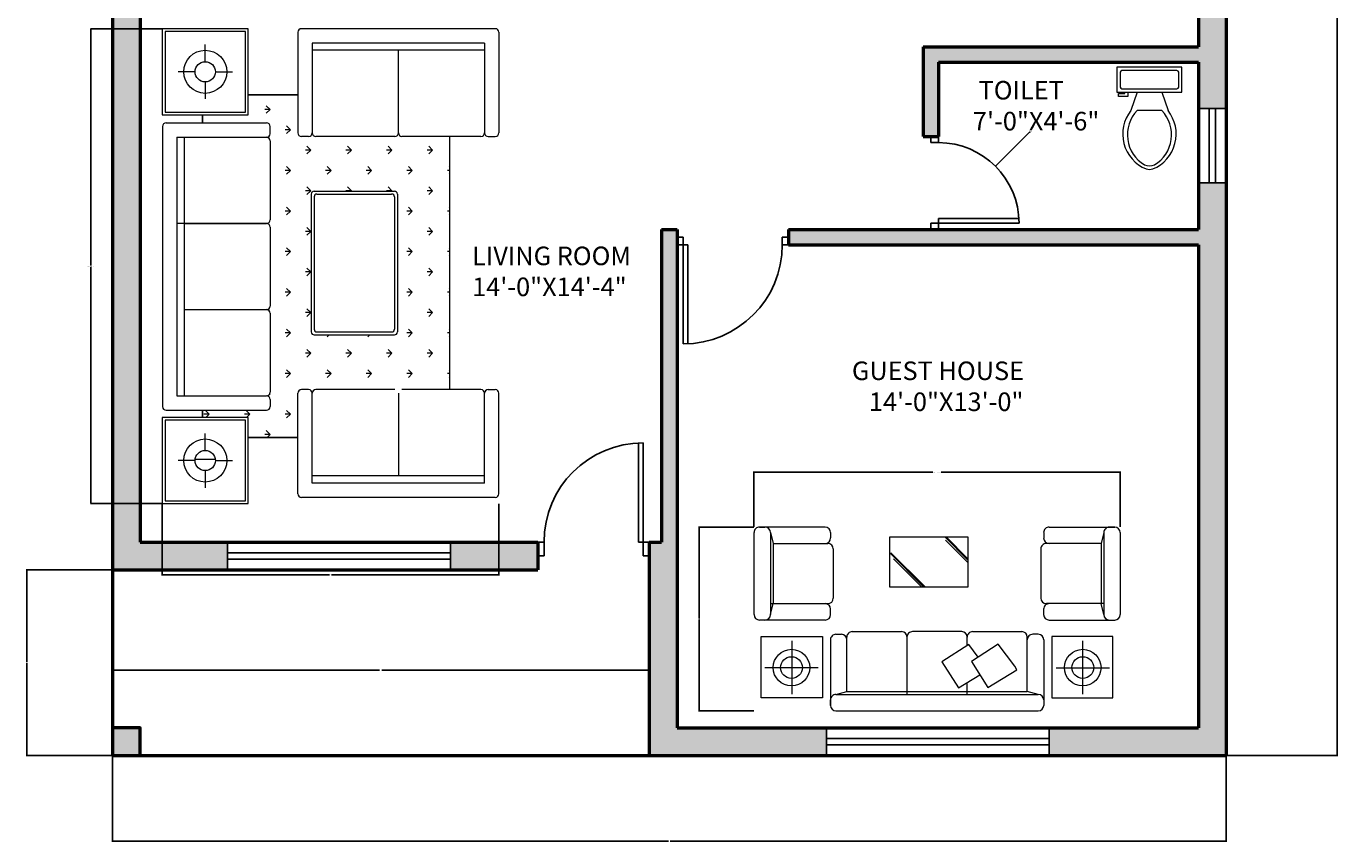
# Model space of a CAD drawing. Units: inches. Extents: x 2831 to 3729, y 3926 to 4974.
# Tile 2 of 8: x 2831 to 3255, y 4438 to 4702. Entities that reach past the tile are written whole.
import ezdxf

# ---------------------------------------------------------------- set-up
doc = ezdxf.new("R2010")
doc.units = ezdxf.units.IN
for name, color, linetype, lineweight in [('A-ANNO-DIMS', 2, 'Continuous', 18), ('A-AREA-IDEN', 7, 'Continuous', 18), ('A-COLS', 7, 'Continuous', 50), ('A-COLS-PATT', 252, 'Continuous', 13), ('A-DOOR', 3, 'Continuous', 25), ('A-FLOR-FIXT', 9, 'Continuous', 18), ('A-FURN', 8, 'Continuous', 18), ('A-GLAZ', 4, 'Continuous', 25), ('A-WALL', 7, 'Continuous', 50), ('A-WALL-PATT', 252, 'Continuous', 13)]:
    doc.layers.add(name, color=color, linetype=linetype, lineweight=lineweight)
doc.styles.get("Standard").update_dxf_attribs({"font": 'arial.ttf'})
doc.dimstyles.get("Standard").update_dxf_attribs({"dimtxt": 0.18, "dimasz": 0.18, "dimexe": 0.18, "dimexo": 0.0625, "dimgap": 0.09, "dimtad": 0, "dimtih": 1, "dimtoh": 1, "dimdec": 4, "dimzin": 0, "dimdsep": 46, "dimtxsty": 'Standard', "dimcen": 0.09, "dimadec": 0, "dimazin": 0, "dimtfac": 1, "dimtdec": 4, "dimtofl": 0, "dimtmove": 0, "dimatfit": 3, "dimfxl": 1, "dimtolj": 1, "dimtzin": 0, "dimarcsym": 0})

# ---------------------------------------------------------------- blocks, each defined once
blk = doc.blocks.new('A$C1C4057EB')
for p, q in [((0, 2345.3, -1028.6), (0, 1745.3, -1028.6)), ((600, 2345.3, -1028.6), (0, 2345.3, -1028.6)), ((20, 2325.3, -1028.6), (20, 1765.3, -1028.6)), ((580, 2325.3, -1028.6), (20, 2325.3, -1028.6)), ((580, 1765.3, -1028.6), (580, 2325.3, -1028.6)), ((600, 1745.3, -1028.6), (600, 2345.3, -1028.6)), ((650.5, 2318, -1028.6), (650.5, 1618, -1028.6)), ((2625.5, 2343, -1028.6), (674.4, 2343, -1028.6)), ((2650.5, 2318, -1028.6), (2650.5, 1618, -1028.6)), ((3306.6, 2345.3, -1028.6), (2706.6, 2345.3, -1028.6)), ((2706.6, 2345.3, -1028.6), (2706.6, 1745.3, -1028.6)), ((3286.6, 2325.3, -1028.6), (2726.6, 2325.3, -1028.6)), ((2726.6, 2325.3, -1028.6), (2726.6, 1765.3, -1028.6)), ((3286.6, 1765.3, -1028.6), (3286.6, 2325.3, -1028.6)), ((3306.6, 1745.3, -1028.6), (3306.6, 2345.3, -1028.6)), ((300, 2115.8, -1028.6), (300, 2234.6, -1028.6)), ((2550.5, 2243, -1028.6), (750.5, 2243, -1028.6)), ((750.5, 2243, -1028.6), (750.5, 1618, -1028.6)), ((2550.5, 2193, -1028.6), (750.5, 2193, -1028.6)), ((1350.5, 2193, -1028.6), (1350.5, 1618, -1028.6)), ((1950.5, 2193, -1028.6), (1950.5, 1618, -1028.6)), ((1952.5, 2243, -1028.6), (1952.5, 1608.2, -1028.6)), ((2550.5, 2243, -1028.6), (2550.5, 1618, -1028.6)), ((3006.6, 2115.8, -1028.6), (3006.6, 2234.6, -1028.6)), ((310, 2115, -1028.6), (310, 1975.5, -1028.6)), ((229.5, 2045.3, -1028.6), (110.6, 2045.3, -1028.6)), ((370.5, 2045.3, -1028.6), (489.4, 2045.3, -1028.6)), ((650.5, 2064.6, -1028.6), (600, 2064.6, -1028.6)), ((600, 2064.6, -1028.6), (650.5, 2064.6, -1028.6)), ((622.9, 2017.7, -1028.6), (600, 2040.6, -1028.6)), ((622.9, 2017.7, -1028.6), (622.9, 2055.2, -1028.6)), ((622.9, 2017.7, -1028.6), (649.4, 2044.2, -1028.6)), ((2706.6, 2064.6, -1028.6), (2650.5, 2064.6, -1028.6)), ((2650.5, 2064.6, -1028.6), (2706.6, 2064.6, -1028.6)), ((2936.1, 2045.3, -1028.6), (2817.3, 2045.3, -1028.6)), ((3077.1, 2045.3, -1028.6), (3196, 2045.3, -1028.6)), ((300, 1974.8, -1028.6), (300, 1855.9, -1028.6)), ((3006.6, 1974.8, -1028.6), (3006.6, 1855.9, -1028.6)), ((0, 1745.3, -1028.6), (600, 1745.3, -1028.6)), ((20, 1765.3, -1028.6), (580, 1765.3, -1028.6)), ((460, 1400, -1028.6), (460, 1745.3, -1028.6)), ((460, 1745.3, -1028.6), (460, 1400, -1028.6)), ((622.9, 1734.8, -1028.6), (600, 1757.7, -1028.6)), ((622.9, 1734.8, -1028.6), (622.9, 1772.3, -1028.6)), ((622.9, 1734.8, -1028.6), (649.4, 1761.4, -1028.6)), ((2706.6, 1745.3, -1028.6), (3306.6, 1745.3, -1028.6)), ((2726.6, 1765.3, -1028.6), (3286.6, 1765.3, -1028.6)), ((2846.6, 1400, -1028.6), (2846.6, 1745.3, -1028.6)), ((2846.6, 1745.3, -1028.6), (2846.6, 1400, -1028.6)), ((481.5, 1593.4, -1028.6), (460, 1614.9, -1028.6)), ((481.5, 1593.4, -1028.6), (481.5, 1630.9, -1028.6)), ((481.5, 1593.4, -1028.6), (508, 1619.9, -1028.6)), ((725.5, 1593, -1028.6), (675.5, 1593, -1028.6)), ((764.3, 1593.4, -1028.6), (748.8, 1608.9, -1028.6)), ((764.3, 1593.4, -1028.6), (764.3, 1595.6, -1028.6)), ((764.3, 1593.4, -1028.6), (765.8, 1594.9, -1028.6)), ((1325.5, 1593, -1028.6), (775.5, 1593, -1028.6)), ((1350.2, 1613.6, -1028.6), (1350.8, 1614.2, -1028.6)), ((1925.5, 1593, -1028.6), (1375.5, 1593, -1028.6)), ((2525.5, 1593, -1028.6), (1975.5, 1593, -1028.6)), ((2575.5, 1593, -1028.6), (2625.5, 1593, -1028.6)), ((2744.2, 1593.4, -1028.6), (2717.7, 1619.9, -1028.6)), ((2744.2, 1593.4, -1028.6), (2744.2, 1630.9, -1028.6)), ((2744.2, 1593.4, -1028.6), (2770.7, 1619.9, -1028.6)), ((622.9, 1452, -1028.6), (596.4, 1478.5, -1028.6)), ((622.9, 1452, -1028.6), (622.9, 1489.5, -1028.6)), ((622.9, 1452, -1028.6), (649.4, 1478.5, -1028.6)), ((905.7, 1452, -1028.6), (879.2, 1478.5, -1028.6)), ((905.7, 1452, -1028.6), (905.7, 1489.5, -1028.6)), ((905.7, 1452, -1028.6), (932.3, 1478.5, -1028.6)), ((1188.6, 1452, -1028.6), (1162.1, 1478.5, -1028.6)), ((1188.6, 1452, -1028.6), (1188.6, 1489.5, -1028.6)), ((1188.6, 1452, -1028.6), (1215.1, 1478.5, -1028.6)), ((1471.4, 1452, -1028.6), (1444.9, 1478.5, -1028.6)), ((1471.4, 1452, -1028.6), (1471.4, 1489.5, -1028.6)), ((1471.4, 1452, -1028.6), (1497.9, 1478.5, -1028.6)), ((1754.3, 1452, -1028.6), (1727.8, 1478.5, -1028.6)), ((1754.3, 1452, -1028.6), (1754.3, 1489.5, -1028.6)), ((1754.3, 1452, -1028.6), (1780.8, 1478.5, -1028.6)), ((2037.1, 1452, -1028.6), (2010.6, 1478.5, -1028.6)), ((2037.1, 1452, -1028.6), (2037.1, 1489.5, -1028.6)), ((2037.1, 1452, -1028.6), (2063.6, 1478.5, -1028.6)), ((2320, 1452, -1028.6), (2293.4, 1478.5, -1028.6)), ((2320, 1452, -1028.6), (2320, 1489.5, -1028.6)), ((2320, 1452, -1028.6), (2346.5, 1478.5, -1028.6)), ((2602.8, 1452, -1028.6), (2576.3, 1478.5, -1028.6)), ((2602.8, 1452, -1028.6), (2602.8, 1489.5, -1028.6)), ((2602.8, 1452, -1028.6), (2629.3, 1478.5, -1028.6)), ((43.5, 25, -1028.6), (43.5, 1375, -1028.6)), ((68.5, 1400, -1028.6), (768.5, 1400, -1028.6)), ((793.5, 1325, -1028.6), (793.5, 1375, -1028.6)), ((2556.6, 1325, -1028.6), (2556.6, 1375, -1028.6)), ((3281.6, 1400, -1028.6), (2581.6, 1400, -1028.6)), ((3306.6, 25, -1028.6), (3306.6, 1375, -1028.6)), ((143.5, 100, -1028.6), (143.5, 1300, -1028.6)), ((143.5, 1300, -1028.6), (768.5, 1300, -1028.6)), ((193.5, 100, -1028.6), (193.5, 1300, -1028.6)), ((1047.2, 1310.6, -1028.6), (1020.7, 1337.1, -1028.6)), ((1047.2, 1310.6, -1028.6), (1047.2, 1348.1, -1028.6)), ((1047.2, 1310.6, -1028.6), (1073.7, 1337.1, -1028.6)), ((1175.1, 1286.9, -1028.6), (1175.1, 726.9, -1028.6)), ((2155.1, 1306.9, -1028.6), (1195.1, 1306.9, -1028.6)), ((2135.1, 1286.9, -1028.6), (1215.1, 1286.9, -1028.6)), ((1330, 1310.6, -1028.6), (1303.5, 1337.1, -1028.6)), ((1330, 1310.6, -1028.6), (1330, 1348.1, -1028.6)), ((1330, 1310.6, -1028.6), (1356.5, 1337.1, -1028.6)), ((1612.9, 1310.6, -1028.6), (1586.3, 1337.1, -1028.6)), ((1612.9, 1310.6, -1028.6), (1612.9, 1348.1, -1028.6)), ((1612.9, 1310.6, -1028.6), (1639.4, 1337.1, -1028.6)), ((1895.7, 1310.6, -1028.6), (1869.2, 1337.1, -1028.6)), ((1895.7, 1310.6, -1028.6), (1895.7, 1348.1, -1028.6)), ((1895.7, 1310.6, -1028.6), (1922.2, 1337.1, -1028.6)), ((2178.5, 1310.6, -1028.6), (2152, 1337.1, -1028.6)), ((2175.1, 1286.9, -1028.6), (2175.1, 726.9, -1028.6)), ((2178.5, 1310.6, -1028.6), (2178.5, 1348.1, -1028.6)), ((2178.5, 1310.6, -1028.6), (2205.1, 1337.1, -1028.6)), ((2461.4, 1310.6, -1028.6), (2434.9, 1337.1, -1028.6)), ((2461.4, 1310.6, -1028.6), (2461.4, 1348.1, -1028.6)), ((2461.4, 1310.6, -1028.6), (2487.9, 1337.1, -1028.6)), ((3206.6, 1300, -1028.6), (2581.6, 1300, -1028.6)), ((3156.6, 100, -1028.6), (3156.6, 1300, -1028.6)), ((3206.6, 100, -1028.6), (3206.6, 1300, -1028.6)), ((793.5, 725, -1028.6), (793.5, 1275, -1028.6)), ((905.7, 1169.2, -1028.6), (879.2, 1195.7, -1028.6)), ((905.7, 1169.2, -1028.6), (905.7, 1206.7, -1028.6)), ((905.7, 1169.2, -1028.6), (932.3, 1195.7, -1028.6)), ((1175.1, 1182.7, -1028.6), (1162.1, 1195.7, -1028.6)), ((1195.1, 1266.9, -1028.6), (1195.1, 746.9, -1028.6)), ((2155.1, 1266.9, -1028.6), (2155.1, 746.9, -1028.6)), ((2320, 1169.2, -1028.6), (2293.4, 1195.7, -1028.6)), ((2320, 1169.2, -1028.6), (2320, 1206.7, -1028.6)), ((2320, 1169.2, -1028.6), (2346.5, 1195.7, -1028.6)), ((2556.6, 725, -1028.6), (2556.6, 1275, -1028.6)), ((1047.2, 1027.7, -1028.6), (1020.7, 1054.2, -1028.6)), ((1047.2, 1027.7, -1028.6), (1047.2, 1065.2, -1028.6)), ((1047.2, 1027.7, -1028.6), (1073.7, 1054.2, -1028.6)), ((2178.5, 1027.7, -1028.6), (2175.1, 1031.2, -1028.6)), ((2178.5, 1027.7, -1028.6), (2178.5, 1065.2, -1028.6)), ((2178.5, 1027.7, -1028.6), (2205.1, 1054.2, -1028.6)), ((2461.4, 1027.7, -1028.6), (2434.9, 1054.2, -1028.6)), ((2461.4, 1027.7, -1028.6), (2461.4, 1065.2, -1028.6)), ((2461.4, 1027.7, -1028.6), (2487.9, 1054.2, -1028.6)), ((905.7, 886.3, -1028.6), (905.7, 923.8, -1028.6)), ((2320, 886.3, -1028.6), (2320, 923.8, -1028.6)), ((905.7, 886.3, -1028.6), (879.2, 912.8, -1028.6)), ((905.7, 886.3, -1028.6), (932.3, 912.8, -1028.6)), ((1175.1, 899.9, -1028.6), (1162.1, 912.8, -1028.6)), ((2320, 886.3, -1028.6), (2293.4, 912.8, -1028.6)), ((2320, 886.3, -1028.6), (2346.5, 912.8, -1028.6)), ((1047.2, 744.9, -1028.6), (1020.7, 771.4, -1028.6)), ((1047.2, 744.9, -1028.6), (1047.2, 782.4, -1028.6)), ((1047.2, 744.9, -1028.6), (1073.7, 771.4, -1028.6)), ((2178.5, 744.9, -1028.6), (2175.1, 748.4, -1028.6)), ((2178.5, 744.9, -1028.6), (2178.5, 782.4, -1028.6)), ((2178.5, 744.9, -1028.6), (2205.1, 771.4, -1028.6)), ((2461.4, 744.9, -1028.6), (2434.9, 771.4, -1028.6)), ((2461.4, 744.9, -1028.6), (2461.4, 782.4, -1028.6)), ((2461.4, 744.9, -1028.6), (2487.9, 771.4, -1028.6)), ((768.5, 700, -1028.6), (193.5, 700, -1028.6)), ((793.5, 125, -1028.6), (793.5, 675, -1028.6)), ((905.7, 603.5, -1028.6), (905.7, 641, -1028.6)), ((1188.6, 603.5, -1028.6), (1188.6, 641, -1028.6)), ((2155.1, 706.9, -1028.6), (1195.1, 706.9, -1028.6)), ((2135.1, 726.9, -1028.6), (1215.1, 726.9, -1028.6)), ((1471.4, 603.5, -1028.6), (1471.4, 641, -1028.6)), ((1754.3, 603.5, -1028.6), (1754.3, 641, -1028.6)), ((2037.1, 603.5, -1028.6), (2037.1, 641, -1028.6)), ((2320, 603.5, -1028.6), (2320, 641, -1028.6)), ((2556.6, 125, -1028.6), (2556.6, 675, -1028.6)), ((2581.6, 700, -1028.6), (3156.6, 700, -1028.6)), ((905.7, 603.5, -1028.6), (879.2, 630, -1028.6)), ((905.7, 603.5, -1028.6), (932.3, 630, -1028.6)), ((1188.6, 603.5, -1028.6), (1162.1, 630, -1028.6)), ((1188.6, 603.5, -1028.6), (1215.1, 630, -1028.6)), ((1471.4, 603.5, -1028.6), (1444.9, 630, -1028.6)), ((1471.4, 603.5, -1028.6), (1497.9, 630, -1028.6)), ((1754.3, 603.5, -1028.6), (1727.8, 630, -1028.6)), ((1754.3, 603.5, -1028.6), (1780.8, 630, -1028.6)), ((2037.1, 603.5, -1028.6), (2010.6, 630, -1028.6)), ((2037.1, 603.5, -1028.6), (2063.6, 630, -1028.6)), ((2320, 603.5, -1028.6), (2293.4, 630, -1028.6)), ((2320, 603.5, -1028.6), (2346.5, 630, -1028.6)), ((1047.2, 462, -1028.6), (1020.7, 488.6, -1028.6)), ((1047.2, 462, -1028.6), (1047.2, 499.5, -1028.6)), ((1047.2, 462, -1028.6), (1073.7, 488.6, -1028.6)), ((1330, 462, -1028.6), (1303.5, 488.6, -1028.6)), ((1330, 462, -1028.6), (1330, 499.5, -1028.6)), ((1330, 462, -1028.6), (1356.5, 488.6, -1028.6)), ((1612.9, 462, -1028.6), (1586.3, 488.6, -1028.6)), ((1612.9, 462, -1028.6), (1612.9, 499.5, -1028.6)), ((1612.9, 462, -1028.6), (1639.4, 488.6, -1028.6)), ((1895.7, 462, -1028.6), (1869.2, 488.6, -1028.6)), ((1895.7, 462, -1028.6), (1895.7, 499.5, -1028.6)), ((1895.7, 462, -1028.6), (1922.2, 488.6, -1028.6)), ((2178.5, 462, -1028.6), (2152, 488.6, -1028.6)), ((2178.5, 462, -1028.6), (2178.5, 499.5, -1028.6)), ((2178.5, 462, -1028.6), (2205.1, 488.6, -1028.6)), ((2461.4, 462, -1028.6), (2434.9, 488.6, -1028.6)), ((2461.4, 462, -1028.6), (2461.4, 499.5, -1028.6)), ((2461.4, 462, -1028.6), (2487.9, 488.6, -1028.6)), ((2556.6, 344.7, -1028.6), (793.5, 344.7, -1028.6)), ((2556.6, 344.7, -1028.6), (793.5, 344.7, -1028.6)), ((881.7, 344.7, -1028.6), (879.2, 347.1, -1028.6)), ((905.7, 344.7, -1028.6), (905.7, 358.1, -1028.6)), ((929.8, 344.7, -1028.6), (932.3, 347.1, -1028.6)), ((1164.6, 344.7, -1028.6), (1162.1, 347.1, -1028.6)), ((1188.6, 344.7, -1028.6), (1188.6, 358.1, -1028.6)), ((1212.6, 344.7, -1028.6), (1215.1, 347.1, -1028.6)), ((1447.4, 344.7, -1028.6), (1444.9, 347.1, -1028.6)), ((1471.4, 344.7, -1028.6), (1471.4, 358.1, -1028.6)), ((1495.5, 344.7, -1028.6), (1497.9, 347.1, -1028.6)), ((1730.2, 344.7, -1028.6), (1727.8, 347.1, -1028.6)), ((1754.3, 344.7, -1028.6), (1754.3, 358.1, -1028.6)), ((1778.3, 344.7, -1028.6), (1780.8, 347.1, -1028.6)), ((2013.1, 344.7, -1028.6), (2010.6, 347.1, -1028.6)), ((2037.1, 344.7, -1028.6), (2037.1, 358.1, -1028.6)), ((2061.1, 344.7, -1028.6), (2063.6, 347.1, -1028.6)), ((2295.9, 344.7, -1028.6), (2293.4, 347.1, -1028.6)), ((2320, 344.7, -1028.6), (2320, 358.1, -1028.6)), ((2344, 344.7, -1028.6), (2346.5, 347.1, -1028.6)), ((143.5, 100, -1028.6), (768.5, 100, -1028.6)), ((3206.6, 100, -1028.6), (2581.6, 100, -1028.6)), ((793.5, 75, -1028.6), (793.5, 25, -1028.6)), ((2556.6, 75, -1028.6), (2556.6, 25, -1028.6)), ((68.5, 0, -1028.6), (768.5, 0, -1028.6)), ((3281.6, 0, -1028.6), (2581.6, 0, -1028.6))]:
    blk.add_line(p, q)
for centre, radius in [((300, 2045.3, -1028.6), 150), ((3006.6, 2045.3, -1028.6), 150), ((300, 2045.3, -1028.6), 70.5), ((3006.6, 2045.3, -1028.6), 70.5)]:
    blk.add_circle(centre, radius)
for centre, radius, start, end in [((675.5, 2318, -1028.6), 25, 90, 180), ((2625.5, 2318, -1028.6), 25, 0, 90), ((675.5, 1618, -1028.6), 25, 180, 270), ((725.5, 1618, -1028.6), 25, 270, 0), ((775.5, 1618, -1028.6), 25, 180, 270), ((1325.5, 1618, -1028.6), 25, 270, 0), ((1375.5, 1618, -1028.6), 25, 180, 270), ((1925.5, 1618, -1028.6), 25, 270, 0), ((1975.5, 1618, -1028.6), 25, 180, 270), ((2525.5, 1618, -1028.6), 25, 270, 0), ((2575.5, 1618, -1028.6), 25, 180, 270), ((2625.5, 1618, -1028.6), 25, 270, 0), ((68.5, 1375, -1028.6), 25, 90, 180), ((768.5, 1375, -1028.6), 25, 0, 90), ((2581.6, 1375, -1028.6), 25, 90, 180), ((3281.6, 1375, -1028.6), 25, 0, 90), ((768.5, 1325, -1028.6), 25, 270, 0), ((768.5, 1275, -1028.6), 25, 0, 90), ((1195.1, 1286.9, -1028.6), 20, 90, 180), ((1215.1, 1266.9, -1028.6), 20, 90, 180), ((2135.1, 1266.9, -1028.6), 20, 0, 90), ((2155.1, 1286.9, -1028.6), 20, 0, 90), ((2581.6, 1325, -1028.6), 25, 180, 270), ((2581.6, 1275, -1028.6), 25, 90, 180), ((1215.1, 746.9, -1028.6), 20, 180, 270), ((2135.1, 746.9, -1028.6), 20, 270, 0), ((1195.1, 726.9, -1028.6), 20, 180, 270), ((2155.1, 726.9, -1028.6), 20, 270, 0), ((2581.6, 725, -1028.6), 25, 180, 270), ((2581.6, 675, -1028.6), 25, 90, 180), ((768.5, 125, -1028.6), 25, 270, 0), ((768.5, 75, -1028.6), 25, 0, 90), ((2581.6, 125, -1028.6), 25, 180, 270), ((2581.6, 75, -1028.6), 25, 90, 180), ((68.5, 25, -1028.6), 25, 180, 270), ((768.5, 25, -1028.6), 25, 270, 0), ((2581.6, 25, -1028.6), 25, 180, 270), ((3281.6, 25, -1028.6), 25, 270, 0)]:
    blk.add_arc(centre, radius, start, end)
blk = doc.blocks.new('A$C780F33EA')
for p, q in [((726, 1649), (726, 1648)), ((2552, 1649), (736, 1649)), ((687, 1011), (687, 1600)), ((2601, 1011), (2601, 1600)), ((2601, 1600), (2601, 1551)), ((338, 1022), (338, 1500)), ((2552, 1502), (736, 1502)), ((736, 1502), (834, 1477)), ((2454, 1477), (834, 1477)), ((834, 1477), (834, 987)), ((1374, 1502), (1374, 1396)), ((1914, 1502), (1914, 987)), ((2552, 1502), (2454, 1477)), ((2454, 1477), (2454, 987)), ((2949, 1022), (2949, 1500)), ((576, 1264), (97, 1264)), ((2712, 1264), (3191, 1264)), ((1374, 1063), (1374, 987)), ((736, 962), (785, 962)), ((2552, 962), (2503, 962)), ((638, 835), (49, 835)), ((1325, 937), (883, 937)), ((1423, 937), (1865, 937)), ((2405, 937), (1963, 937)), ((2649, 835), (3238, 835)), ((0, 49), (0, 785)), ((147, 49), (147, 785)), ((147, 785), (172, 687)), ((687, 785), (687, 736)), ((2600, 785), (2600, 736)), ((3140, 785), (3116, 687)), ((3140, 49), (3140, 785)), ((3288, 49), (3288, 785)), ((147, 687), (663, 687)), ((172, 147), (172, 687)), ((172, 687), (663, 687)), ((656, 691), (656, 687)), ((712, 196), (712, 638)), ((2576, 196), (2576, 638)), ((3116, 687), (2625, 687)), ((3140, 687), (2625, 687)), ((2631, 691), (2631, 687)), ((3116, 147), (3116, 687)), ((2058, 230), (1754, 534)), ((2068, 232), (1765, 535)), ((2036, 285), (1782, 539)), ((1568, 118), (1368, 319)), ((1575, 89), (1368, 297)), ((1563, 89), (1368, 285)), ((147, 49), (172, 147)), ((172, 147), (663, 147)), ((656, 147), (656, 144)), ((3116, 147), (2625, 147)), ((2631, 147), (2631, 144)), ((3140, 49), (3116, 147)), ((638, 0), (49, 0)), ((49, 0), (98, 0)), ((687, 49), (687, 98)), ((2600, 49), (2600, 98)), ((2649, 0), (3238, 0)), ((3238, 0), (3189, 0))]:
    blk.add_line(p, q)
for points in [[(615, 1531), (65, 1531), (65, 981), (615, 981)], [(2672, 1531), (3222, 1531), (3222, 981), (2672, 981)], [(946, 1249), (1096, 1051), (1336, 1206), (1187, 1440), (928, 1281)], [(1368, 539), (2068, 539), (2068, 89), (1368, 89)]]:
    blk.add_lwpolyline(points, close=True)
blk.add_lwpolyline([(1275, 1166), (1360, 1054), (1600, 1209), (1451, 1443), (1260, 1325)])
for centre, radius in [((336, 1261), 164), ((2951, 1261), 164), ((336, 1261), 97.9), ((2951, 1261), 97.9)]:
    blk.add_circle(centre, radius)
for centre, start, end in [((736, 1600), 90, 180), ((2552, 1600), 0, 90), ((2552, 1600), 0, 90), ((736, 1551), 180, 270), ((2552, 1551), 270, 0), ((736, 1011), 180, 270), ((785, 1011), 270, 0), ((883, 987), 180, 270), ((1325, 987), 270, 0), ((1423, 987), 180, 270), ((1865, 987), 270, 0), ((1963, 987), 180, 270), ((2405, 987), 270, 0), ((2503, 1011), 180, 270), ((2552, 1011), 270, 0), ((49, 785), 90, 180), ((98, 785), 0, 90), ((638, 785), 0, 90), ((2649, 785), 90, 180), ((3189, 785), 90, 180), ((3238, 785), 0, 90), ((638, 736), 270, 0), ((2649, 736), 180, 270), ((663, 638), 0, 90), ((2625, 638), 90, 180), ((638, 98), 0, 90), ((663, 196), 270, 0), ((2625, 196), 180, 270), ((2649, 98), 90, 180), ((49, 49), 180, 270), ((49, 49), 180, 270), ((98, 49), 270, 0), ((638, 49), 270, 0), ((2649, 49), 180, 270), ((3189, 49), 180, 270), ((3238, 49), 270, 0), ((3238, 49), 270, 0)]:
    blk.add_arc(centre, 49.1, start, end)
blk = doc.blocks.new('*U8')
for p, q in [((9.5, -6), (9.5, -2)), ((-8, -8.5), (-8, -8)), ((-7, -8), (-7, -9.5)), ((-4, -8), (-6, -14)), ((4, -8), (6, -14)), ((-10, -8.5), (-8, -8.5)), ((-10, -9.5), (-10, -8.5)), ((-7, -9.5), (-10, -9.5)), ((4, -14), (-4, -14))]:
    blk.add_line(p, q)
blk.add_lwpolyline([(10.5, -8), (10.5, 0), (-10.5, 0), (-10.5, -8)], close=True)
for points in [[(-9.5, -2), (-9.5, -6)], [(8.5, -1), (-8.5, -1)], [(-8.5, -7), (8.5, -7)]]:
    blk.add_lwpolyline(points)
for centre, radius, start, end in [((-8.62, -1.88), 0.884, 81.8699, 188.1301), ((8.62, -1.88), 0.884, 351.8699, 98.1301), ((-8.62, -6.12), 0.884, 171.8699, 278.1301), ((8.62, -6.12), 0.884, 261.8699, 8.1301), ((3.52, -21.58), 12.17, 141.4691, 247.9714), ((4.2, -21.82), 11.33, 136.3677, 238.9468), ((-3.52, -21.58), 12.17, 292.0284, 38.5307), ((-4.2, -21.82), 11.33, 301.053, 43.6321), ((0, -27.88), 4, 245.7318, 294.2682), ((0, -29), 4, 254.8605, 285.1395)]:
    blk.add_arc(centre, radius, start, end)
blk = doc.blocks.new('DOOR-SWING-32IN')
for p, q in [((-32, 2.5), (-34, 2.5)), ((-34, 0), (-32, 0)), ((-32, 0), (-32, 2.5)), ((0, 0), (0, 2.5)), ((0, 2.5), (2, 2.5)), ((2, 0), (0, 0)), ((-1.5, 0), (-1.5, -31.96)), ((0, 0), (-1.5, 0)), ((0, 0), (0, -32))]:
    blk.add_line(p, q)
blk.add_arc((0, 0), 32, 180, 270)
blk = doc.blocks.new('DOOR-SWING-26IN')
for p, q in [((-1.5, 25.96), (-1.5, 0)), ((0, 26), (0, 0)), ((-26, 0), (-28, 0)), ((-26, -2.5), (-26, 0)), ((0, 0), (-1.5, 0)), ((0, -2.5), (0, 0)), ((0, 0), (2, 0)), ((-28, -2.5), (-26, -2.5)), ((2, -2.5), (0, -2.5))]:
    blk.add_line(p, q)
blk.add_arc((0, 0), 26, 90, 180)
blk = doc.blocks.new('DOOR-SWING-32IN-DEEP-JAMB')
for p, q in [((0, 0), (0, 32)), ((1.5, 0), (1.5, 31.96)), ((0, 0), (-2, 0)), ((0, -4.5), (0, 0)), ((0, 0), (1.5, 0)), ((32, -4.5), (32, 0)), ((32, 0), (34, 0)), ((-2, -4.5), (0, -4.5)), ((34, -4.5), (32, -4.5))]:
    blk.add_line(p, q)
blk.add_arc((0, 0), 32, 0, 90)
blk = doc.blocks.new('WINDOW-72IN-PLAN')
for p, q in [((0, 0), (0, 9)), ((72, 0), (72, 9)), ((72, 5.5), (0, 5.5)), ((72, 3.5), (0, 3.5))]:
    blk.add_line(p, q)
blk = doc.blocks.new('WINDOW-24IN-PLAN')
for p, q in [((0, 24), (9, 24)), ((3.5, 0), (3.5, 24)), ((5.5, 0), (5.5, 24)), ((0, 0), (9, 0))]:
    blk.add_line(p, q)
blk = doc.blocks.new('*D43')
at = {"layer": 'A-ANNO-DIMS', "color": 0, "lineweight": -2, "transparency": 16777216}
for p, q in [((2874.53, 4700.95), (2851.4, 4700.95)), ((2851.58, 4700.77), (2851.58, 4624.43)), ((2851.58, 4547.72), (2851.58, 4624.06)), ((2874.53, 4547.54), (2851.4, 4547.54))]:
    blk.add_line(p, q, dxfattribs=at)
at = {"layer": 'A-ANNO-DIMS', "color": 0, "transparency": 16777216}
for points in [[(2851.55, 4700.77), (2851.61, 4700.77), (2851.58, 4700.95)], [(2851.55, 4547.72), (2851.61, 4547.72), (2851.58, 4547.54)]]:
    blk.add_solid(points, dxfattribs=at)
at = {"layer": 'Defpoints', "color": 0, "transparency": 16777216}
for p in [(2851.58, 4700.95), (2874.59, 4700.95), (2874.59, 4547.54)]:
    blk.add_point(p, dxfattribs=at)
at = {"layer": 'A-ANNO-DIMS', "color": 0, "transparency": 16777216, "insert": (2851.58, 4624.25), "char_height": 0.18, "attachment_point": 5}
blk.add_mtext('\\A1;LIVING ROOM SET 153', dxfattribs=at)
blk = doc.blocks.new('*D44')
at = {"layer": 'A-ANNO-DIMS', "color": 0, "lineweight": -2, "transparency": 16777216}
for p, q in [((2874.59, 4547.48), (2874.59, 4524.35)), ((2983.41, 4547.48), (2983.41, 4524.35)), ((2874.77, 4524.53), (2928.72, 4524.53)), ((2983.23, 4524.53), (2929.28, 4524.53))]:
    blk.add_line(p, q, dxfattribs=at)
at = {"layer": 'A-ANNO-DIMS', "color": 0, "transparency": 16777216}
for points in [[(2874.77, 4524.56), (2874.77, 4524.5), (2874.59, 4524.53)], [(2983.23, 4524.56), (2983.23, 4524.5), (2983.41, 4524.53)]]:
    blk.add_solid(points, dxfattribs=at)
at = {"layer": 'Defpoints', "color": 0, "transparency": 16777216}
for p in [(2874.59, 4547.54), (2983.41, 4547.54), (2874.59, 4524.53)]:
    blk.add_point(p, dxfattribs=at)
at = {"layer": 'A-ANNO-DIMS', "color": 0, "transparency": 16777216, "insert": (2929, 4524.53), "char_height": 0.18, "attachment_point": 5}
blk.add_mtext('\\A1;109', dxfattribs=at)
blk = doc.blocks.new('*D45')
at = {"layer": 'A-ANNO-DIMS', "color": 0, "lineweight": -2, "transparency": 16777216}
for p, q in [((3065.85, 4540.02), (3065.85, 4557.89)), ((3066.03, 4557.71), (3123.68, 4557.71)), ((3184.01, 4557.71), (3126.36, 4557.71)), ((3184.19, 4540.02), (3184.19, 4557.89))]:
    blk.add_line(p, q, dxfattribs=at)
at = {"layer": 'A-ANNO-DIMS', "color": 0, "transparency": 16777216}
for points in [[(3066.03, 4557.74), (3066.03, 4557.68), (3065.85, 4557.71)], [(3184.01, 4557.74), (3184.01, 4557.68), (3184.19, 4557.71)]]:
    blk.add_solid(points, dxfattribs=at)
at = {"layer": 'Defpoints', "color": 0, "transparency": 16777216}
for p in [(3065.85, 4557.71), (3065.85, 4539.96), (3184.19, 4539.96)]:
    blk.add_point(p, dxfattribs=at)
at = {"layer": 'A-ANNO-DIMS', "color": 0, "transparency": 16777216, "insert": (3125.02, 4557.71), "char_height": 0.18, "attachment_point": 5}
blk.add_mtext('\\A1;GUEST SEATING 118', dxfattribs=at)
blk = doc.blocks.new('*D46')
at = {"layer": 'A-ANNO-DIMS', "color": 0, "lineweight": -2, "transparency": 16777216}
for p, q in [((3065.79, 4539.96), (3047.92, 4539.96)), ((3048.1, 4539.78), (3048.1, 4510.46)), ((3048.1, 4480.78), (3048.1, 4510.1)), ((3065.79, 4480.6), (3047.92, 4480.6))]:
    blk.add_line(p, q, dxfattribs=at)
at = {"layer": 'A-ANNO-DIMS', "color": 0, "transparency": 16777216}
for points in [[(3048.07, 4539.78), (3048.13, 4539.78), (3048.1, 4539.96)], [(3048.07, 4480.78), (3048.13, 4480.78), (3048.1, 4480.6)]]:
    blk.add_solid(points, dxfattribs=at)
at = {"layer": 'Defpoints', "color": 0, "transparency": 16777216}
for p in [(3065.85, 4539.96), (3048.1, 4480.6), (3065.85, 4480.6)]:
    blk.add_point(p, dxfattribs=at)
at = {"layer": 'A-ANNO-DIMS', "color": 0, "transparency": 16777216, "insert": (3048.1, 4510.28), "char_height": 0.18, "attachment_point": 5}
blk.add_mtext('\\A1;59', dxfattribs=at)
blk = doc.blocks.new('*D47')
at = {"layer": 'A-ANNO-DIMS', "color": 0, "lineweight": -2, "transparency": 16777216}
for p, q in [((2858.49, 4466.08), (2858.49, 4438.31)), ((3218.49, 4466.08), (3218.49, 4438.31)), ((2858.67, 4438.49), (3038.2, 4438.49)), ((3218.31, 4438.49), (3038.78, 4438.49))]:
    blk.add_line(p, q, dxfattribs=at)
at = {"layer": 'A-ANNO-DIMS', "color": 0, "transparency": 16777216}
for points in [[(2858.67, 4438.52), (2858.67, 4438.46), (2858.49, 4438.49)], [(3218.31, 4438.52), (3218.31, 4438.46), (3218.49, 4438.49)]]:
    blk.add_solid(points, dxfattribs=at)
at = {"layer": 'Defpoints', "color": 0, "transparency": 16777216}
for p in [(2858.49, 4466.14), (3218.49, 4466.14), (3218.49, 4438.49)]:
    blk.add_point(p, dxfattribs=at)
at = {"layer": 'A-ANNO-DIMS', "color": 0, "transparency": 16777216, "insert": (3038.49, 4438.49), "char_height": 0.18, "attachment_point": 5}
blk.add_mtext('\\A1;360', dxfattribs=at)
blk = doc.blocks.new('*D48')
at = {"layer": 'A-ANNO-DIMS', "color": 0, "lineweight": -2, "transparency": 16777216}
for p, q in [((3218.55, 4946.14), (3254.48, 4946.14)), ((3254.3, 4945.96), (3254.3, 4706.32)), ((3254.3, 4466.32), (3254.3, 4705.96)), ((3218.55, 4466.14), (3254.48, 4466.14))]:
    blk.add_line(p, q, dxfattribs=at)
at = {"layer": 'A-ANNO-DIMS', "color": 0, "transparency": 16777216}
for points in [[(3254.27, 4945.96), (3254.33, 4945.96), (3254.3, 4946.14)], [(3254.27, 4466.32), (3254.33, 4466.32), (3254.3, 4466.14)]]:
    blk.add_solid(points, dxfattribs=at)
at = {"layer": 'Defpoints', "color": 0, "transparency": 16777216}
for p in [(3218.49, 4946.14), (3254.3, 4946.14), (3218.49, 4466.14)]:
    blk.add_point(p, dxfattribs=at)
at = {"layer": 'A-ANNO-DIMS', "color": 0, "transparency": 16777216, "insert": (3254.3, 4706.14), "char_height": 0.18, "attachment_point": 5}
blk.add_mtext('\\A1;480', dxfattribs=at)
blk = doc.blocks.new('*D49')
at = {"layer": 'A-ANNO-DIMS', "color": 0, "lineweight": -2, "transparency": 16777216}
for p, q in [((2858.49, 4466.2), (2858.49, 4493.97)), ((2858.67, 4493.79), (2944.86, 4493.79)), ((3031.81, 4493.79), (2945.63, 4493.79)), ((3031.99, 4466.2), (3031.99, 4493.97))]:
    blk.add_line(p, q, dxfattribs=at)
at = {"layer": 'A-ANNO-DIMS', "color": 0, "transparency": 16777216}
for points in [[(2858.67, 4493.82), (2858.67, 4493.76), (2858.49, 4493.79)], [(3031.81, 4493.82), (3031.81, 4493.76), (3031.99, 4493.79)]]:
    blk.add_solid(points, dxfattribs=at)
at = {"layer": 'Defpoints', "color": 0, "transparency": 16777216}
for p in [(3031.99, 4493.79), (2858.49, 4466.14), (3031.99, 4466.14)]:
    blk.add_point(p, dxfattribs=at)
at = {"layer": 'A-ANNO-DIMS', "color": 0, "transparency": 16777216, "insert": (2945.24, 4493.79), "char_height": 0.18, "attachment_point": 5}
blk.add_mtext('\\A1;173.5', dxfattribs=at)
blk = doc.blocks.new('*D50')
at = {"layer": 'A-ANNO-DIMS', "color": 0, "lineweight": -2, "transparency": 16777216}
for p, q in [((2858.43, 4526.14), (2830.66, 4526.14)), ((2830.84, 4525.96), (2830.84, 4496.32)), ((2830.84, 4466.32), (2830.84, 4495.96)), ((2858.43, 4466.14), (2830.66, 4466.14))]:
    blk.add_line(p, q, dxfattribs=at)
at = {"layer": 'A-ANNO-DIMS', "color": 0, "transparency": 16777216}
for points in [[(2830.81, 4525.96), (2830.87, 4525.96), (2830.84, 4526.14)], [(2830.81, 4466.32), (2830.87, 4466.32), (2830.84, 4466.14)]]:
    blk.add_solid(points, dxfattribs=at)
at = {"layer": 'Defpoints', "color": 0, "transparency": 16777216}
for p in [(2830.84, 4526.14), (2858.49, 4526.14), (2858.49, 4466.14)]:
    blk.add_point(p, dxfattribs=at)
at = {"layer": 'A-ANNO-DIMS', "color": 0, "transparency": 16777216, "insert": (2830.84, 4496.14), "char_height": 0.18, "attachment_point": 5}
blk.add_mtext('\\A1;60', dxfattribs=at)
blk = doc.blocks.new('*D79')
at = {"layer": 'A-ANNO-DIMS', "color": 0, "lineweight": -2, "transparency": 16777216}
for p, q in [((3154.91, 4667.56), (3144, 4656.65)), ((3155.09, 4667.56), (3154.91, 4667.56)), ((3125.4, 4638.14), (3125.58, 4638.14)), ((3125.49, 4638.05), (3125.49, 4638.23))]:
    blk.add_line(p, q, dxfattribs=at)
at = {"layer": 'A-ANNO-DIMS', "color": 0, "transparency": 16777216}
blk.add_solid([(3143.98, 4656.67), (3144.02, 4656.63), (3143.88, 4656.53)], dxfattribs=at)
at = {"layer": 'Defpoints', "color": 0, "transparency": 16777216}
for p in [(3143.88, 4656.53), (3125.49, 4638.14)]:
    blk.add_point(p, dxfattribs=at)
at = {"layer": 'A-ANNO-DIMS', "color": 0, "transparency": 16777216, "insert": (3155.39, 4667.56), "char_height": 0.18, "attachment_point": 5}
blk.add_mtext('\\A1;R26', dxfattribs=at)

msp = doc.modelspace()

# ---------------------------------------------------------------- hatches: boundary and pattern name
at = {"layer": 'A-COLS-PATT'}
h = msp.add_hatch(color=256, dxfattribs=at)
h.dxf.hatch_style = 1
h.paths.add_polyline_path([(2867.4912, 4475.1405), (2858.4912, 4475.1405), (2858.4912, 4466.1405), (2867.4912, 4466.1405)])
at = {"layer": 'A-WALL-PATT'}
h = msp.add_hatch(color=256, dxfattribs=at)
h.dxf.hatch_style = 1
h.paths.add_polyline_path([(2867.4912, 4707.1405), (2999.9912, 4707.1405), (2999.9912, 4712.1405), (2867.4912, 4712.1405), (2867.4912, 4788.1405), (2999.9912, 4788.1405), (2999.9912, 4793.1405), (2867.4912, 4793.1405), (2867.4912, 4937.1405), (2915.7412, 4937.1405), (2915.7412, 4946.1405), (2858.4912, 4946.1405), (2858.4912, 4526.1405), (2895.7412, 4526.1405), (2895.7412, 4535.1405), (2867.4912, 4535.1405)])
h.paths.add_polyline_path([(3071.1162, 4946.1405), (2987.7412, 4946.1405), (2987.7412, 4937.1405), (3035.9912, 4937.1405), (3035.9912, 4788.1405), (3101.2412, 4788.1405), (3101.2412, 4793.1405), (3040.9912, 4793.1405), (3040.9912, 4937.1405), (3071.1162, 4937.1405)])
h = msp.add_hatch(color=256, dxfattribs=at)
h.dxf.hatch_style = 1
h.paths.add_polyline_path([(3218.4912, 4946.1405), (3119.1162, 4946.1405), (3119.1162, 4937.1405), (3149.2412, 4937.1405), (3149.2412, 4829.1405), (3154.2412, 4829.1405), (3154.2412, 4937.1405), (3209.4912, 4937.1405), (3209.4912, 4793.1405), (3149.2412, 4793.1405), (3149.2412, 4788.1405), (3209.4912, 4788.1405), (3209.4912, 4695.1405), (3120.4912, 4695.1405), (3120.4912, 4666.1405), (3125.4912, 4666.1405), (3125.4912, 4690.1405), (3209.4912, 4690.1405), (3209.4912, 4675.1405), (3218.4912, 4675.1405)])
h = msp.add_hatch(color=256, dxfattribs=at)
h.dxf.hatch_style = 1
h.paths.add_polyline_path([(3218.4912, 4651.1405), (3209.4912, 4651.1405), (3209.4912, 4636.1405), (3076.9912, 4636.1405), (3076.9912, 4631.1405), (3209.4912, 4631.1405), (3209.4912, 4475.1405), (3161.2412, 4475.1405), (3161.2412, 4466.1405), (3218.4912, 4466.1405)])
h = msp.add_hatch(color=256, dxfattribs=at)
h.dxf.hatch_style = 1
h.paths.add_polyline_path([(3040.9912, 4636.1405), (3035.9912, 4636.1405), (3035.9912, 4535.1405), (3031.9912, 4535.1405), (3031.9912, 4466.1405), (3089.2412, 4466.1405), (3089.2412, 4475.1405), (3040.9912, 4475.1405)])
h = msp.add_hatch(color=256, dxfattribs=at)
h.dxf.hatch_style = 1
h.paths.add_polyline_path([(2995.9912, 4535.1405), (2967.7412, 4535.1405), (2967.7412, 4526.1405), (2995.9912, 4526.1405)])

# ---------------------------------------------------------------- linework, layer by layer
at = {"layer": 'A-COLS'}
msp.add_lwpolyline([(2858.4912, 4466.1405), (2867.4912, 4466.1405), (2867.4912, 4475.1405), (2858.4912, 4475.1405)], close=True, dxfattribs=at)
at = {"layer": 'A-WALL'}
for p, q in [((2858.4912, 4946.1405), (2858.4912, 4466.1405)), ((3218.4912, 4946.1405), (3218.4912, 4466.1405)), ((3209.4912, 4788.1405), (3209.4912, 4695.1405)), ((2867.4912, 4707.1405), (2867.4912, 4535.1405)), ((3120.4912, 4695.1405), (3209.4912, 4695.1405)), ((3120.4912, 4695.1405), (3120.4912, 4666.1405)), ((3125.4912, 4690.1405), (3209.4912, 4690.1405)), ((3125.4912, 4690.1405), (3125.4912, 4666.1405)), ((3209.4912, 4690.1405), (3209.4912, 4636.1405)), ((3120.4912, 4666.1405), (3125.4912, 4666.1405)), ((3035.9912, 4636.1405), (3040.9912, 4636.1405)), ((3035.9912, 4636.1405), (3035.9912, 4535.1405)), ((3040.9912, 4636.1405), (3040.9912, 4475.1405)), ((3076.9912, 4636.1405), (3076.9912, 4631.1405)), ((3076.9912, 4636.1405), (3209.4912, 4636.1405)), ((3076.9912, 4631.1405), (3209.4912, 4631.1405)), ((3209.4912, 4631.1405), (3209.4912, 4475.1405)), ((2867.4912, 4535.1405), (2995.9912, 4535.1405)), ((2995.9912, 4535.1405), (2995.9912, 4526.1405)), ((3031.9912, 4535.1405), (3031.9912, 4466.1405)), ((3031.9912, 4535.1405), (3035.9912, 4535.1405)), ((2858.4912, 4526.1405), (2995.9912, 4526.1405)), ((3040.9912, 4475.1405), (3209.4912, 4475.1405)), ((2858.4912, 4466.1405), (3218.4912, 4466.1405))]:
    msp.add_line(p, q, dxfattribs=at)

# ---------------------------------------------------------------- block references
at = {"layer": 'A-DOOR', "rotation": 269.9999999999977}
msp.add_blockref('DOOR-SWING-26IN', (3125.4912, 4638.1405), dxfattribs=at)
at = {"layer": 'A-DOOR', "extrusion": (0, 0, -1), "zscale": -1}
for name, p in [('DOOR-SWING-32IN', (-3042.9912, 4631.1405)), ('DOOR-SWING-32IN-DEEP-JAMB', (-3029.9912, 4535.1405))]:
    msp.add_blockref(name, p, dxfattribs=at)
at = {"layer": 'A-FLOR-FIXT'}
msp.add_blockref('*U8', (3193.6494, 4688.5016), dxfattribs=at)
at = {"layer": 'A-FURN'}
for name, p, xscale, yscale, zscale, rotation in [('A$C1C4057EB', (2983.4058, 4547.538, -1414.4284), 0.0463962252557528, 0.0463962252557528, 0.0463962252557528, 90), ('A$C780F33EA', (3184.1908, 4539.9621), 0.0359954658623315, 0.0359954658623315, 0.0359954658623315, 180)]:
    msp.add_blockref(name, p, dxfattribs=dict(at, xscale=xscale, yscale=yscale, zscale=zscale, rotation=rotation))
at = {"layer": 'A-GLAZ'}
for name, p in [('WINDOW-24IN-PLAN', (3209.4912, 4651.1405)), ('WINDOW-72IN-PLAN', (3089.2412, 4466.1405))]:
    msp.add_blockref(name, p, dxfattribs=at)
at = {"layer": 'A-GLAZ', "rotation": 180}
msp.add_blockref('WINDOW-72IN-PLAN', (2967.7412, 4535.1405), dxfattribs=at)

# ---------------------------------------------------------------- texts
at = {"layer": 'A-AREA-IDEN', "attachment_point": 1}
for s, width, insert, char_height in [(' TOILET\\P7\'-0"X4\'-6"', 76.299971, (3136.5985, 4684.0842), 6), ('{\\H2.4x;LIVING ROOM\\P14\'-0"X14\'-4"}', 77.245421, (2974.7619, 4630.5638), 2.5), ('GUEST HOUSE\\P   14\'-0"X13\'-0"', 76.299971, (3097.4927, 4593.446), 6)]:
    msp.add_mtext_dynamic_manual_height_columns(s, width=width, gutter_width=12.5, heights=[0], dxfattribs=dict(at, insert=insert, char_height=char_height))

# ---------------------------------------------------------------- dimensions: what is measured, and where the dimension line sits
at = {"layer": 'A-ANNO-DIMS'}
for base, p1, p2, angle, picture, middle in [((3254.2994, 4946.1405), (3218.4912, 4466.1405), (3218.4912, 4946.1405), 90, '*D48', (3254.2994, 4706.1405)), ((2874.5948, 4524.5256), (2983.4058, 4547.538), (2874.5948, 4547.538), 180, '*D44', (2929.0003, 4524.5256)), ((3048.1031, 4480.5971), (3065.8537, 4539.9621), (3065.8537, 4480.5971), 270, '*D46', (3048.1031, 4510.2796)), ((2830.8412, 4526.1405), (2858.4912, 4466.1405), (2858.4912, 4526.1405), 90, '*D50', (2830.8412, 4496.1405))]:
    dim = msp.add_linear_dim(base=base, p1=p1, p2=p2, angle=angle, dimstyle='Standard', override={"dimdec": 0, "dimlfac": 1, "dimrnd": 0, "dimzin": 0, "dimdsep": 46, "dimlunit": 2}, dxfattribs=at)
    dim.commit()
    dim.dimension.update_dxf_attribs({"geometry": picture, "text_midpoint": middle})
for base, p1, p2, angle, text, picture, middle in [((2851.5824, 4700.9535), (2874.5948, 4547.538), (2874.5948, 4700.9535), 90, 'LIVING ROOM SET <>', '*D43', (2851.5824, 4624.2457)), ((3065.8537, 4557.7126), (3184.1908, 4539.9621), (3065.8537, 4539.9621), 180, 'GUEST SEATING <>', '*D45', (3125.0222, 4557.7126))]:
    dim = msp.add_linear_dim(base=base, p1=p1, p2=p2, angle=angle, text=text, dimstyle='Standard', override={"dimdec": 0, "dimlfac": 1, "dimrnd": 0, "dimzin": 0, "dimdsep": 46, "dimlunit": 2}, dxfattribs=at)
    dim.commit()
    dim.dimension.update_dxf_attribs({"geometry": picture, "text_midpoint": middle})
dim = msp.add_radius_dim(center=(3125.4912, 4638.1405), mpoint=(3143.8761, 4656.5251), dimstyle='Standard', override={"dimdec": 0, "dimlfac": 1, "dimrnd": 0, "dimzin": 0, "dimdsep": 46, "dimlunit": 2}, dxfattribs=at)
dim.commit()
dim.dimension.update_dxf_attribs({"geometry": '*D79', "text_midpoint": (3155.3921, 4667.5559), "dimtype": 164})
for base, p2, override, picture, middle in [((3031.9912, 4493.7905), (3031.9912, 4466.1405), {"dimdec": 1, "dimlfac": 1, "dimrnd": 0, "dimzin": 0, "dimdsep": 46, "dimlunit": 2}, '*D49', (2945.2412, 4493.7905)), ((3218.4912, 4438.4905), (3218.4912, 4466.1405), {"dimdec": 0, "dimlfac": 1, "dimrnd": 0, "dimzin": 0, "dimdsep": 46, "dimlunit": 2}, '*D47', (3038.4912, 4438.4905))]:
    dim = msp.add_linear_dim(base=base, p1=(2858.4912, 4466.1405), p2=p2, dimstyle='Standard', override=override, dxfattribs=at)
    dim.commit()
    dim.dimension.update_dxf_attribs({"geometry": picture, "text_midpoint": middle})

doc.saveas('drawing.dxf')
